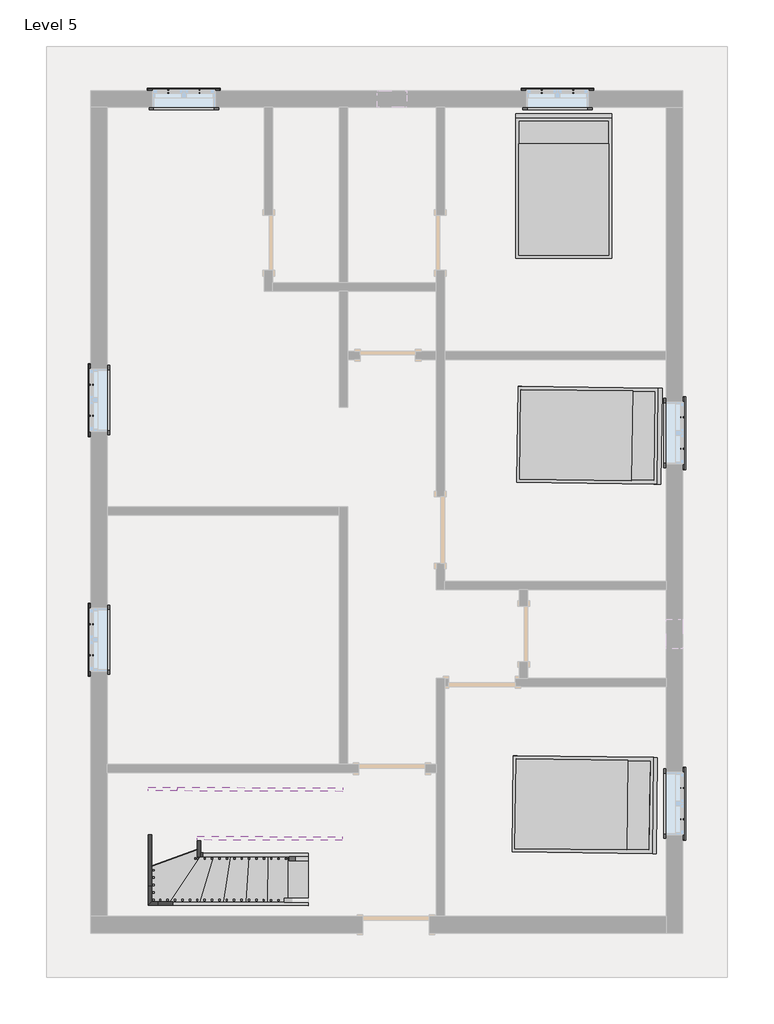
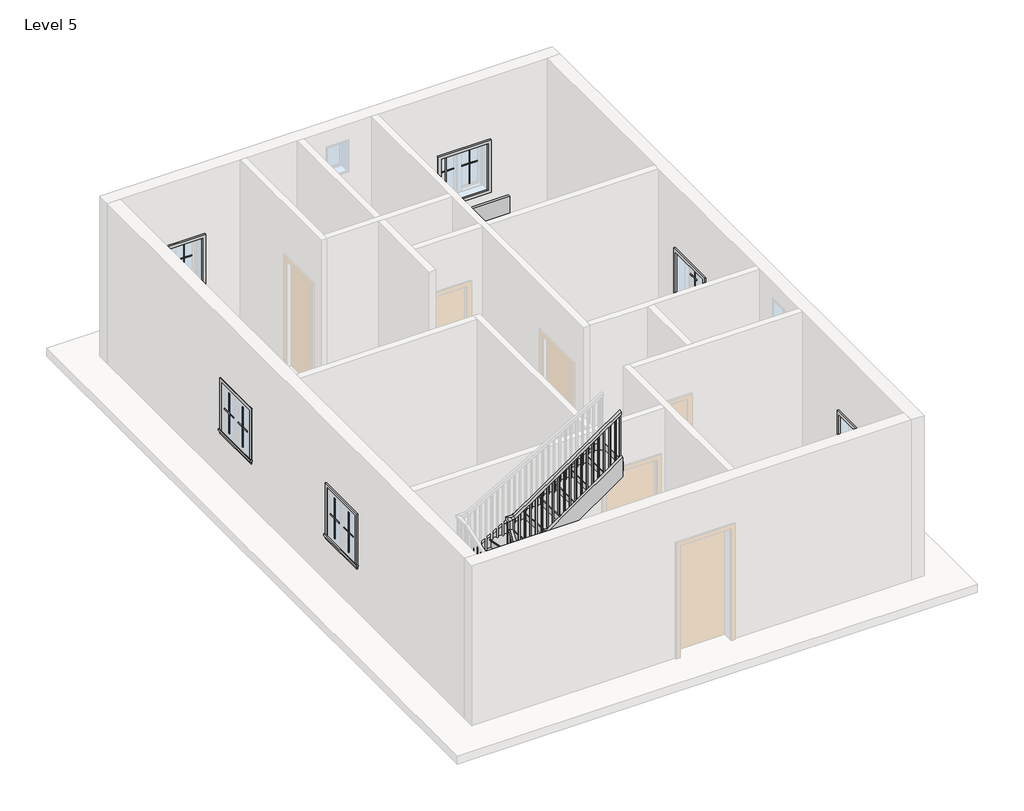
# One storey, part 3 of 3: 24 proxies, 9 members, 3 furniture elements, 1 railing, 1 stair flight.
"""IFC4 building model written with IfcOpenShell, lengths in millimetres."""

from ifc_helpers import new_model, si_unit, frame, origin, place, context, project, spatial, polyline, outline, extrude, faceted_brep, transform, mapped, element, save
from components import muntin_pattern_2x2_muntin_pattern_2x2_b3fe6957, muntin_pattern_2x2_muntin_pattern_2x2_3e0ecaf2, trim_window_exterior_flat_with_sill_41619996, trim_window_interior_flat_picture_frame_51c85655, bed_17739_bed_17739_15c61121, stair_flight_765c7f0f

model = new_model("IFC4")

# Units and contexts
model_context = context("Model", 3, world=origin())
ifc_project = project(units=[si_unit("LENGTHUNIT", "METRE", prefix="MILLI")], contexts=[model_context])

# Site, building, storey
site = spatial("IfcSite", under=ifc_project)
building = spatial("IfcBuilding", under=site)
storey = spatial("IfcBuildingStorey", under=building, Name="Level 5", Elevation=9601.2)

# Proxies
placement = place(None, origin())
muntin_pattern_2x2_muntin_pattern_2x2_shape = muntin_pattern_2x2_muntin_pattern_2x2_b3fe6957(model_context)
element("IfcBuildingElementProxy", 1, Name="Muntin Pattern_2x2 : Muntin Pattern_2x2", ObjectType="Muntin Pattern_2x2 : Muntin Pattern_2x2", at=placement, inside=storey, context=model_context, shape_type="MappedRepresentation", body=[
    mapped(muntin_pattern_2x2_muntin_pattern_2x2_shape, transform((873.7257686, 6321.6571212, 10585.45), x_axis=(1.0, 0.0, 0.0), y_axis=(0.0, 1.0, 0.0), z_axis=(0.0, 0.0, 1.0))),
])
element("IfcBuildingElementProxy", 2, Name="Muntin Pattern_2x2 : Muntin Pattern_2x2", ObjectType="Muntin Pattern_2x2 : Muntin Pattern_2x2", at=placement, inside=storey, context=model_context, shape_type="MappedRepresentation", body=[
    mapped(muntin_pattern_2x2_muntin_pattern_2x2_shape, transform((2802.5382686, 1840.1446212, 10585.45), x_axis=(0.0, -1.0, 0.0), y_axis=(1.0, 0.0, 0.0), z_axis=(0.0, 0.0, 1.0))),
])
element("IfcBuildingElementProxy", 3, Name="Muntin Pattern_2x2 : Muntin Pattern_2x2", ObjectType="Muntin Pattern_2x2 : Muntin Pattern_2x2", at=placement, inside=storey, context=model_context, shape_type="MappedRepresentation", body=[
    mapped(muntin_pattern_2x2_muntin_pattern_2x2_shape, transform((2802.5382686, -3255.7303788, 10585.45), x_axis=(0.0, -1.0, 0.0), y_axis=(1.0, 0.0, 0.0), z_axis=(0.0, 0.0, 1.0))),
])
element("IfcBuildingElementProxy", 4, Name="Muntin Pattern_2x2 : Muntin Pattern_2x2", ObjectType="Muntin Pattern_2x2 : Muntin Pattern_2x2", at=placement, inside=storey, context=model_context, shape_type="MappedRepresentation", body=[
    mapped(muntin_pattern_2x2_muntin_pattern_2x2_shape, transform((-4263.4242314, 6321.6571212, 10585.45), x_axis=(1.0, 0.0, 0.0), y_axis=(0.0, 1.0, 0.0), z_axis=(0.0, 0.0, 1.0))),
])
element("IfcBuildingElementProxy", 5, Name="Muntin Pattern_2x2 : Muntin Pattern_2x2", ObjectType="Muntin Pattern_2x2 : Muntin Pattern_2x2", at=placement, inside=storey, context=model_context, shape_type="MappedRepresentation", body=[
    mapped(muntin_pattern_2x2_muntin_pattern_2x2_shape, transform((-5319.1117314, 1863.8332318, 10585.45), x_axis=(0.0, 1.0, 0.0), y_axis=(-1.0, 0.0, 0.0), z_axis=(0.0, 0.0, 1.0))),
])
element("IfcBuildingElementProxy", 6, Name="Muntin Pattern_2x2 : Muntin Pattern_2x2", ObjectType="Muntin Pattern_2x2 : Muntin Pattern_2x2", at=placement, inside=storey, context=model_context, shape_type="MappedRepresentation", body=[
    mapped(muntin_pattern_2x2_muntin_pattern_2x2_shape, transform((-5319.1117314, -1431.8167682, 10585.45), x_axis=(0.0, 1.0, 0.0), y_axis=(-1.0, 0.0, 0.0), z_axis=(0.0, 0.0, 1.0))),
])
muntin_pattern_2x2_muntin_pattern_2x2_2_shape = muntin_pattern_2x2_muntin_pattern_2x2_3e0ecaf2(model_context)
element("IfcBuildingElementProxy", 7, Name="Muntin Pattern_2x2 : Muntin Pattern_2x2", ObjectType="Muntin Pattern_2x2 : Muntin Pattern_2x2", at=placement, inside=storey, context=model_context, shape_type="MappedRepresentation", body=[
    mapped(muntin_pattern_2x2_muntin_pattern_2x2_2_shape, transform((1302.3507686, 6321.6571212, 10585.45), x_axis=(-1.0, 0.0, 0.0), y_axis=(0.0, -1.0, 0.0), z_axis=(0.0, 0.0, 1.0))),
])
element("IfcBuildingElementProxy", 8, Name="Muntin Pattern_2x2 : Muntin Pattern_2x2", ObjectType="Muntin Pattern_2x2 : Muntin Pattern_2x2", at=placement, inside=storey, context=model_context, shape_type="MappedRepresentation", body=[
    mapped(muntin_pattern_2x2_muntin_pattern_2x2_2_shape, transform((2802.5382686, 1411.5196212, 10585.45), x_axis=(0.0, 1.0, 0.0), y_axis=(-1.0, 0.0, 0.0), z_axis=(0.0, 0.0, 1.0))),
])
element("IfcBuildingElementProxy", 9, Name="Muntin Pattern_2x2 : Muntin Pattern_2x2", ObjectType="Muntin Pattern_2x2 : Muntin Pattern_2x2", at=placement, inside=storey, context=model_context, shape_type="MappedRepresentation", body=[
    mapped(muntin_pattern_2x2_muntin_pattern_2x2_2_shape, transform((2802.5382686, -3684.3553788, 10585.45), x_axis=(0.0, 1.0, 0.0), y_axis=(-1.0, 0.0, 0.0), z_axis=(0.0, 0.0, 1.0))),
])
element("IfcBuildingElementProxy", 10, Name="Muntin Pattern_2x2 : Muntin Pattern_2x2", ObjectType="Muntin Pattern_2x2 : Muntin Pattern_2x2", at=placement, inside=storey, context=model_context, shape_type="MappedRepresentation", body=[
    mapped(muntin_pattern_2x2_muntin_pattern_2x2_2_shape, transform((-3834.7992314, 6321.6571212, 10585.45), x_axis=(-1.0, 0.0, 0.0), y_axis=(0.0, -1.0, 0.0), z_axis=(0.0, 0.0, 1.0))),
])
element("IfcBuildingElementProxy", 11, Name="Muntin Pattern_2x2 : Muntin Pattern_2x2", ObjectType="Muntin Pattern_2x2 : Muntin Pattern_2x2", at=placement, inside=storey, context=model_context, shape_type="MappedRepresentation", body=[
    mapped(muntin_pattern_2x2_muntin_pattern_2x2_2_shape, transform((-5319.1117314, 2292.4582318, 10585.45), x_axis=(0.0, -1.0, 0.0), y_axis=(1.0, 0.0, 0.0), z_axis=(0.0, 0.0, 1.0))),
])
element("IfcBuildingElementProxy", 12, Name="Muntin Pattern_2x2 : Muntin Pattern_2x2", ObjectType="Muntin Pattern_2x2 : Muntin Pattern_2x2", at=placement, inside=storey, context=model_context, shape_type="MappedRepresentation", body=[
    mapped(muntin_pattern_2x2_muntin_pattern_2x2_2_shape, transform((-5319.1117314, -1003.1917682, 10585.45), x_axis=(0.0, -1.0, 0.0), y_axis=(1.0, 0.0, 0.0), z_axis=(0.0, 0.0, 1.0))),
])
trim_window_exterior_flat_with_sill_shape = trim_window_exterior_flat_with_sill_41619996(model_context)
element("IfcBuildingElementProxy", 13, Name="Trim-Window-Exterior-Flat : with Sill", ObjectType="Trim-Window-Exterior-Flat : with Sill", at=placement, inside=storey, context=model_context, shape_type="MappedRepresentation", body=[
    mapped(trim_window_exterior_flat_with_sill_shape, transform((1088.0382686, 6331.1821212, 11430.0), x_axis=(-1.0, 0.0, 0.0), y_axis=(0.0, 0.0, 1.0), z_axis=(0.0, 1.0, 0.0))),
])
element("IfcBuildingElementProxy", 14, Name="Trim-Window-Exterior-Flat : with Sill", ObjectType="Trim-Window-Exterior-Flat : with Sill", at=placement, inside=storey, context=model_context, shape_type="MappedRepresentation", body=[
    mapped(trim_window_exterior_flat_with_sill_shape, transform((2812.0632686, 1625.8321212, 11430.0), x_axis=(0.0, 1.0, 0.0), y_axis=(0.0, 0.0, 1.0), z_axis=(1.0, 0.0, 0.0))),
])
element("IfcBuildingElementProxy", 15, Name="Trim-Window-Exterior-Flat : with Sill", ObjectType="Trim-Window-Exterior-Flat : with Sill", at=placement, inside=storey, context=model_context, shape_type="MappedRepresentation", body=[
    mapped(trim_window_exterior_flat_with_sill_shape, transform((2812.0632686, -3470.0428788, 11430.0), x_axis=(0.0, 1.0, 0.0), y_axis=(0.0, 0.0, 1.0), z_axis=(1.0, 0.0, 0.0))),
])
element("IfcBuildingElementProxy", 16, Name="Trim-Window-Exterior-Flat : with Sill", ObjectType="Trim-Window-Exterior-Flat : with Sill", at=placement, inside=storey, context=model_context, shape_type="MappedRepresentation", body=[
    mapped(trim_window_exterior_flat_with_sill_shape, transform((-4049.1117314, 6331.1821212, 11430.0), x_axis=(-1.0, 0.0, 0.0), y_axis=(0.0, 0.0, 1.0), z_axis=(0.0, 1.0, 0.0))),
])
element("IfcBuildingElementProxy", 17, Name="Trim-Window-Exterior-Flat : with Sill", ObjectType="Trim-Window-Exterior-Flat : with Sill", at=placement, inside=storey, context=model_context, shape_type="MappedRepresentation", body=[
    mapped(trim_window_exterior_flat_with_sill_shape, transform((-5328.6367314, 2078.1457318, 11430.0), x_axis=(0.0, -1.0, 0.0), y_axis=(0.0, 0.0, 1.0), z_axis=(-1.0, 0.0, 0.0))),
])
element("IfcBuildingElementProxy", 18, Name="Trim-Window-Exterior-Flat : with Sill", ObjectType="Trim-Window-Exterior-Flat : with Sill", at=placement, inside=storey, context=model_context, shape_type="MappedRepresentation", body=[
    mapped(trim_window_exterior_flat_with_sill_shape, transform((-5328.6367314, -1217.5042682, 11430.0), x_axis=(0.0, -1.0, 0.0), y_axis=(0.0, 0.0, 1.0), z_axis=(-1.0, 0.0, 0.0))),
])
trim_window_interior_flat_picture_frame_shape = trim_window_interior_flat_picture_frame_51c85655(model_context)
element("IfcBuildingElementProxy", 19, Name="Trim-Window-Interior-Flat : Picture Frame", ObjectType="Trim-Window-Interior-Flat : Picture Frame", at=placement, inside=storey, context=model_context, shape_type="MappedRepresentation", body=[
    mapped(trim_window_interior_flat_picture_frame_shape, transform((1088.0382686, 6102.5821212, 11430.0), x_axis=(1.0, 0.0, 0.0), y_axis=(0.0, 0.0, 1.0), z_axis=(0.0, -1.0, 0.0))),
])
element("IfcBuildingElementProxy", 20, Name="Trim-Window-Interior-Flat : Picture Frame", ObjectType="Trim-Window-Interior-Flat : Picture Frame", at=placement, inside=storey, context=model_context, shape_type="MappedRepresentation", body=[
    mapped(trim_window_interior_flat_picture_frame_shape, transform((2583.4632686, 1625.8321212, 11430.0), x_axis=(0.0, -1.0, 0.0), y_axis=(0.0, 0.0, 1.0), z_axis=(-1.0, 0.0, 0.0))),
])
element("IfcBuildingElementProxy", 21, Name="Trim-Window-Interior-Flat : Picture Frame", ObjectType="Trim-Window-Interior-Flat : Picture Frame", at=placement, inside=storey, context=model_context, shape_type="MappedRepresentation", body=[
    mapped(trim_window_interior_flat_picture_frame_shape, transform((2583.4632686, -3470.0428788, 11430.0), x_axis=(0.0, -1.0, 0.0), y_axis=(0.0, 0.0, 1.0), z_axis=(-1.0, 0.0, 0.0))),
])
element("IfcBuildingElementProxy", 22, Name="Trim-Window-Interior-Flat : Picture Frame", ObjectType="Trim-Window-Interior-Flat : Picture Frame", at=placement, inside=storey, context=model_context, shape_type="MappedRepresentation", body=[
    mapped(trim_window_interior_flat_picture_frame_shape, transform((-4049.1117314, 6102.5821212, 11430.0), x_axis=(1.0, 0.0, 0.0), y_axis=(0.0, 0.0, 1.0), z_axis=(0.0, -1.0, 0.0))),
])
element("IfcBuildingElementProxy", 23, Name="Trim-Window-Interior-Flat : Picture Frame", ObjectType="Trim-Window-Interior-Flat : Picture Frame", at=placement, inside=storey, context=model_context, shape_type="MappedRepresentation", body=[
    mapped(trim_window_interior_flat_picture_frame_shape, transform((-5100.0367314, 2078.1457318, 11430.0), x_axis=(0.0, 1.0, 0.0), y_axis=(0.0, 0.0, 1.0), z_axis=(1.0, 0.0, 0.0))),
])
element("IfcBuildingElementProxy", 24, Name="Trim-Window-Interior-Flat : Picture Frame", ObjectType="Trim-Window-Interior-Flat : Picture Frame", at=placement, inside=storey, context=model_context, shape_type="MappedRepresentation", body=[
    mapped(trim_window_interior_flat_picture_frame_shape, transform((-5100.0367314, -1217.5042682, 11430.0), x_axis=(0.0, 1.0, 0.0), y_axis=(0.0, 0.0, 1.0), z_axis=(1.0, 0.0, 0.0))),
])

# Furniture
bed_17739_bed_17739_shape = bed_17739_bed_17739_15c61121(model_context)
element("IfcFurniture", 25, ObjectType="Bed_17739 : Bed_17739", at=placement, inside=storey, context=model_context, shape_type="MappedRepresentation", body=[
    mapped(bed_17739_bed_17739_shape, transform((1173.7632686, 4997.6821212, 9601.2), x_axis=(1.0, 0.0, 0.0), y_axis=(0.0, 1.0, 0.0), z_axis=(0.0, 0.0, 1.0))),
])
element("IfcFurniture", 26, ObjectType="Bed_17739 : Bed_17739", at=placement, inside=storey, context=model_context, shape_type="MappedRepresentation", body=[
    mapped(bed_17739_bed_17739_shape, transform((1503.3372561, 1596.4447738, 9601.2), x_axis=(-0.012740965827000846, -0.9999188306006619, 0.0), y_axis=(0.9999188306006619, -0.012740965827000846, 0.0), z_axis=(0.0, 0.0, 1.0))),
])
element("IfcFurniture", 27, ObjectType="Bed_17739 : Bed_17739", at=placement, inside=storey, context=model_context, shape_type="MappedRepresentation", body=[
    mapped(bed_17739_bed_17739_shape, transform((1438.6034215, -3483.9063624, 9601.2), x_axis=(-0.012740965827007402, -0.9999188306006618, 0.0), y_axis=(0.9999188306006618, -0.012740965827007402, 0.0), z_axis=(0.0, 0.0, 1.0))),
])

# Members
element("IfcMember", 28, ObjectType="Stringer - 2\" Width", at=placement, inside=storey, context=model_context, shape_type="SweptSolid", body=[
    extrude(outline(polyline([(-105.6436802, -202.41926), (0.0, 0.0), (2328.0658822, 0.0), (2168.9891534, -304.7999999), (90.5236019, -304.7999999), (-105.6436802, -202.41926)])), frame((-2342.1993001, -4876.8012848, 9829.5290257), z_axis=(0.0033835818014385675, 0.9999942756707125, 0.0), x_axis=(-0.8865193579369285, 0.002999627936996439, 0.46268178074713046)), (0.0, 0.0, 1.0), 50.8),
])
element("IfcMember", 29, ObjectType="Stringer - 2\" Width", at=placement, inside=storey, context=model_context, shape_type="SweptSolid", body=[
    extrude(outline(polyline([(-4405.9028852, -4819.0182441), (-4406.0747712, -4869.8179533), (-4542.6986856, -4869.3556725), (-4491.7270905, -4818.7278493), (-4405.9028852, -4819.0182441)])), frame((0.0, 0.0, 10562.8681426), z_axis=(0.0, 0.0, 1.0), x_axis=(1.0, 0.0, 0.0)), (0.0, 0.0, 1.0), 343.8145513),
])
element("IfcMember", 30, ObjectType="Stringer - 2\" Width", at=placement, inside=storey, context=model_context, shape_type="SweptSolid", body=[
    extrude(outline(polyline([(-4491.7270905, -4818.7278493), (-4542.6986856, -4869.3556725), (-4541.8102896, -4606.7963526), (-4491.0105804, -4606.9682386), (-4491.7270905, -4818.7278493)])), frame((0.0, 0.0, 10562.8681426), z_axis=(0.0, 0.0, 1.0), x_axis=(1.0, 0.0, 0.0)), (0.0, 0.0, 1.0), 343.8145513),
])
element("IfcMember", 31, ObjectType="Stringer - 2\" Width", at=placement, inside=storey, context=model_context, shape_type="SweptSolid", body=[
    extrude(outline(polyline([(109.7110974, -325.8403301), (0.0, 0.0), (1383.9510961, 0.0), (1489.930143, -314.7561954), (1457.0104275, -325.8403301), (109.7110974, -325.8403301)])), frame((-4491.0105804, -4606.9682386, 10562.8681426), z_axis=(-0.9999942756707125, 0.003383581801438881, 0.0), x_axis=(0.0032066921171017425, 0.9477157489074123, 0.3190996339680272)), (0.0, 0.0, 1.0), 50.8),
])
element("IfcMember", 32, ObjectType="Stringer - 2\" Width", at=placement, inside=storey, context=model_context, shape_type="SweptSolid", body=[
    extrude(outline(polyline([(-4537.3723845, -3295.2041032), (-4537.2004986, -3244.404394), (-4139.0142012, -3245.7516976), (-4139.1860871, -3296.5514068), (-4537.3723845, -3295.2041032)])), frame((0.0, 0.0, 11014.9918365), z_axis=(0.0, 0.0, 1.0), x_axis=(1.0, 0.0, 0.0)), (0.0, 0.0, 1.0), 321.6135804),
])
element("IfcMember", 33, ObjectType="Stringer - 2\" Width", at=placement, inside=storey, context=model_context, shape_type="SweptSolid", body=[
    extrude(outline(polyline([(-111.9549294, -160.635527), (0.0, 0.0), (1800.2454177, 0.0), (1587.8150598, -304.8000001), (94.8955973, -304.8), (-111.9549294, -160.635527)])), frame((-2339.9228929, -4204.0248458, 9797.0000989), z_axis=(0.0033835818014388334, 0.9999942756707125, 0.0), x_axis=(-0.82040105359797, 0.0027759099650580487, 0.5717817814334475)), (0.0, 0.0, 1.0), 50.8),
])
element("IfcMember", 34, ObjectType="Stringer - 2\" Width", at=placement, inside=storey, context=model_context, shape_type="SweptSolid", body=[
    extrude(outline(polyline([(438.5777673, -304.8), (2.5808594, -1.7936294), (3.8273846, 0.0), (400.5684618, 0.0), (819.8223258, -291.370396), (810.4891046, -304.8000001), (438.5777673, -304.8)])), frame((-3816.8461303, -4199.0275266, 10487.0862902), z_axis=(-0.9999942756707126, 0.00338358180143736, 0.0), x_axis=(0.0019309727886813012, 0.5706856959500531, 0.8211663094538725)), (0.0, 0.0, 1.0), 50.8),
])
element("IfcMember", 35, ObjectType="Stringer - 2\" Width", at=placement, inside=storey, context=model_context, shape_type="SweptSolid", body=[
    extrude(outline(polyline([(213.8292849, -304.8), (0.0, 0.0), (2440.5867528, 0.0), (2654.4160377, -304.8), (213.8292849, -304.8)])), frame((-3866.8723527, -3970.2569493, 10954.2535021), z_axis=(0.003383581801438697, 0.9999942756707126, 0.0), x_axis=(0.8186346554264393, -0.0027699331781375542, 0.5743079560697587)), (0.0, 0.0, 1.0), 50.8),
])
element("IfcMember", 36, ObjectType="Stringer - 2\" Width", at=placement, inside=storey, context=model_context, shape_type="SweptSolid", body=[
    extrude(outline(polyline([(162.5062199, -277.5374274), (0.0, 0.0), (2633.4595913, 1e-07), (2795.9658112, -277.5374274), (162.5062199, -277.5374274)])), frame((-4139.1860871, -3296.5514068, 11014.9918365), z_axis=(0.003383581801438589, 0.9999942756707125, 0.0), x_axis=(0.8629481327443966, -0.002919872311849943, 0.5052840731100098)), (0.0, 0.0, 1.0), 50.8),
])

# Railing
element("IfcRailing", 37, ObjectType="Handrail - Rectangular", at=placement, inside=storey, context=model_context, shape_type="SolidModel", body=[
    faceted_brep([(-2340.0947789, -4254.824555, 10684.9333333), (-2340.0947789, -4254.824555, 10623.5023206), (-2339.9228929, -4204.0248458, 10623.5023206), (-2339.9228929, -4204.0248458, 10684.9333333), (-3791.6181617, -4249.9131788, 11671.9092848), (-3842.4178709, -4249.7412929, 11645.0199762), (-3842.2459849, -4198.9415837, 11645.0199762), (-3791.4462757, -4199.1134696, 11671.9092848), (-1868.5796854, -3875.4177931, 13563.6), (-1868.7515713, -3926.2175023, 13563.6), (-1868.7515713, -3926.2175023, 13501.938507), (-1868.5796854, -3875.4177931, 13501.938507), (-3774.5418549, -3868.9687773, 12190.645528), (-3790.329017, -3868.9153598, 12241.445528), (-3774.7137409, -3919.7684865, 12190.645528), (-3790.500903, -3919.715069, 12241.445528), (-3791.6181617, -4249.9131788, 11888.2182666), (-3842.4178709, -4249.7412929, 11837.4182666), (-3842.2459849, -4198.9415837, 11837.4182666), (-3791.4462757, -4199.1134696, 11888.2182666), (-3918.6174347, -4249.4834639, 11888.2182666), (-3918.6174347, -4249.4834639, 11837.4182666), (-3867.6458395, -4198.8556407, 11837.4182666), (-3867.6458395, -4198.8556407, 11888.2182666), (-3918.1877198, -4122.4841909, 11888.2182666), (-3918.0978567, -4095.9257757, 11837.4182666), (-3867.2981475, -4096.0976616, 11837.4182666), (-3867.3880106, -4122.6560769, 11888.2182666), (-3917.7580049, -3995.4849179, 12070.959003), (-3917.586119, -3944.6852087, 12055.0400838), (-3866.7864097, -3944.8570947, 12055.0400838), (-3866.9582957, -3995.6568039, 12070.959003), (-3917.7580049, -3995.4849179, 12241.445528), (-3917.586119, -3944.6852087, 12190.645528), (-3866.7864097, -3944.8570947, 12190.645528), (-3866.9582957, -3995.6568039, 12241.445528), (-3917.32829, -3868.4856449, 12241.445528), (-3917.32829, -3868.4856449, 12190.645528), (-3866.7004668, -3919.4572401, 12190.645528), (-3866.7004668, -3919.4572401, 12241.445528)], [[[0, 1, 2, 3]], [[1, 0, 4, 5]], [[2, 1, 5, 6]], [[3, 2, 6, 7]], [[0, 3, 7, 4]], [[8, 9, 10, 11]], [[12, 13, 8, 11]], [[14, 12, 11, 10]], [[15, 14, 10, 9]], [[13, 15, 9, 8]], [[5, 4, 16, 17]], [[6, 5, 17, 18]], [[7, 6, 18, 19]], [[4, 7, 19, 16]], [[17, 16, 20, 21]], [[18, 17, 21, 22]], [[19, 18, 22, 23]], [[16, 19, 23, 20]], [[21, 20, 24, 25]], [[22, 21, 25, 26]], [[23, 22, 26, 27]], [[20, 23, 27, 24]], [[25, 24, 28, 29]], [[26, 25, 29, 30]], [[27, 26, 30, 31]], [[24, 27, 31, 28]], [[29, 28, 32, 33]], [[30, 29, 33, 34]], [[31, 30, 34, 35]], [[28, 31, 35, 32]], [[33, 32, 36, 37]], [[34, 33, 37, 38]], [[35, 34, 38, 39]], [[32, 35, 39, 36]], [[37, 36, 13, 12]], [[38, 37, 12, 14]], [[39, 38, 14, 15]], [[36, 39, 15, 13]]]),
    extrude(outline(polyline([(222.0468824, -19.0499999), (235.1531175, 0.0), (1186.7159363, 0.0), (1186.7159363, -19.0499999), (222.0468824, -19.0499999)])), frame((-1971.1826027, -3909.9958257, 13666.582603), z_axis=(0.0033835818014386967, 0.9999942756707125, 0.0), x_axis=(0.0, 0.0, -1.0)), (0.0, 0.0, 1.0), 19.05),
    extrude(outline(polyline([(222.0468825, -19.0499999), (235.1531175, 0.0), (1116.8160159, 0.0), (1116.8160159, -19.0499999), (222.0468825, -19.0499999)])), frame((-2072.7820211, -3909.6520537, 13596.6826826), z_axis=(0.0033835818014386967, 0.9999942756707125, 0.0), x_axis=(0.0, 0.0, -1.0)), (0.0, 0.0, 1.0), 19.05),
    extrude(outline(polyline([(222.0468825, -19.0499999), (235.1531176, 0.0), (1216.2494289, 0.0), (1216.2494289, -19.0499999), (222.0468825, -19.0499999)])), frame((-2174.3814395, -3909.3082818, 13526.7827622), z_axis=(0.0033835818014386967, 0.9999942756707125, 0.0), x_axis=(0.0, 0.0, -1.0)), (0.0, 0.0, 1.0), 19.05),
    extrude(outline(polyline([(222.0468825, -19.05), (235.1531175, 0.0), (1146.3495084, 0.0), (1146.3495084, -19.05), (222.0468825, -19.05)])), frame((-2275.980858, -3908.9645099, 13456.8828417), z_axis=(0.0033835818014386967, 0.9999942756707125, 0.0), x_axis=(0.0, 0.0, -1.0)), (0.0, 0.0, 1.0), 19.05),
    extrude(outline(polyline([(222.0468825, -19.05), (235.1531176, 0.0), (1076.449588, 0.0), (1076.449588, -19.05), (222.0468825, -19.05)])), frame((-2377.5802764, -3908.620738, 13386.9829213), z_axis=(0.0033835818014386967, 0.9999942756707125, 0.0), x_axis=(0.0, 0.0, -1.0)), (0.0, 0.0, 1.0), 19.05),
    extrude(outline(polyline([(222.0468824, -19.05), (235.1531175, 0.0), (1175.8830008, 0.0), (1175.8830008, -19.05), (222.0468824, -19.05)])), frame((-2479.1796948, -3908.2769661, 13317.0830008), z_axis=(0.0033835818014386967, 0.9999942756707125, 0.0), x_axis=(0.0, 0.0, -1.0)), (0.0, 0.0, 1.0), 19.05),
    extrude(outline(polyline([(222.0468825, -19.05), (235.1531176, 0.0), (1105.9830804, 0.0), (1105.9830804, -19.05), (222.0468825, -19.05)])), frame((-2580.7791132, -3907.9331942, 13247.1830804), z_axis=(0.0033835818014386967, 0.9999942756707125, 0.0), x_axis=(0.0, 0.0, -1.0)), (0.0, 0.0, 1.0), 19.05),
    extrude(outline(polyline([(222.0468824, -19.05), (235.1531175, 0.0), (1036.0831599, 0.0), (1036.0831599, -19.05), (222.0468824, -19.05)])), frame((-2682.3785316, -3907.5894223, 13177.2831599), z_axis=(0.0033835818014386967, 0.9999942756707125, 0.0), x_axis=(0.0, 0.0, -1.0)), (0.0, 0.0, 1.0), 19.05),
    extrude(outline(polyline([(222.0468825, -19.05), (235.1531176, 0.0), (1135.5165728, 0.0), (1135.5165728, -19.05), (222.0468825, -19.05)])), frame((-2783.97795, -3907.2456504, 13107.3832395), z_axis=(0.0033835818014386967, 0.9999942756707125, 0.0), x_axis=(0.0, 0.0, -1.0)), (0.0, 0.0, 1.0), 19.05),
    extrude(outline(polyline([(222.0468824, -19.0499999), (235.1531175, 0.0), (1065.6166523, 0.0), (1065.6166523, -19.0499999), (222.0468824, -19.0499999)])), frame((-2885.5773684, -3906.9018785, 13037.483319), z_axis=(0.0033835818014386967, 0.9999942756707125, 0.0), x_axis=(0.0, 0.0, -1.0)), (0.0, 0.0, 1.0), 19.05),
    extrude(outline(polyline([(222.0468825, -19.0499999), (235.1531176, 0.0), (995.7167319, 0.0), (995.7167319, -19.0499999), (222.0468825, -19.0499999)])), frame((-2987.1767868, -3906.5581065, 12967.5833986), z_axis=(0.0033835818014386967, 0.9999942756707125, 0.0), x_axis=(0.0, 0.0, -1.0)), (0.0, 0.0, 1.0), 19.05),
    extrude(outline(polyline([(222.0468824, -19.0499999), (235.1531175, 0.0), (1095.1501448, 0.0), (1095.1501448, -19.0499999), (222.0468824, -19.0499999)])), frame((-3088.7762052, -3906.2143346, 12897.6834781), z_axis=(0.0033835818014386967, 0.9999942756707125, 0.0), x_axis=(0.0, 0.0, -1.0)), (0.0, 0.0, 1.0), 19.05),
    extrude(outline(polyline([(222.0468825, -19.0499999), (235.1531176, 0.0), (1025.2502244, 0.0), (1025.2502244, -19.0499999), (222.0468825, -19.0499999)])), frame((-3190.3756236, -3905.8705627, 12827.7835577), z_axis=(0.0033835818014386967, 0.9999942756707125, 0.0), x_axis=(0.0, 0.0, -1.0)), (0.0, 0.0, 1.0), 19.05),
    extrude(outline(polyline([(222.0468824, -19.0499999), (235.1531175, 0.0), (1124.6836372, 0.0), (1124.6836372, -19.0499999), (222.0468824, -19.0499999)])), frame((-3291.975042, -3905.5267908, 12757.8836372), z_axis=(0.0033835818014386967, 0.9999942756707125, 0.0), x_axis=(0.0, 0.0, -1.0)), (0.0, 0.0, 1.0), 19.05),
    extrude(outline(polyline([(222.0468825, -19.0499999), (235.1531176, 0.0), (1054.7837168, 0.0), (1054.7837168, -19.0499999), (222.0468825, -19.0499999)])), frame((-3393.5744604, -3905.1830189, 12687.9837168), z_axis=(0.0033835818014386967, 0.9999942756707125, 0.0), x_axis=(0.0, 0.0, -1.0)), (0.0, 0.0, 1.0), 19.05),
    extrude(outline(polyline([(222.0468824, -19.05), (235.1531175, 0.0), (984.8837963, 0.0), (984.8837963, -19.05), (222.0468824, -19.05)])), frame((-3495.1738789, -3904.839247, 12618.0837963), z_axis=(0.0033835818014386967, 0.9999942756707125, 0.0), x_axis=(0.0, 0.0, -1.0)), (0.0, 0.0, 1.0), 19.05),
    extrude(outline(polyline([(222.0468825, -19.05), (235.1531176, 0.0), (1084.3172092, 0.0), (1084.3172092, -19.05), (222.0468825, -19.05)])), frame((-3596.7732973, -3904.4954751, 12548.1838759), z_axis=(0.0033835818014386967, 0.9999942756707125, 0.0), x_axis=(0.0, 0.0, -1.0)), (0.0, 0.0, 1.0), 19.05),
    extrude(outline(polyline([(222.0468824, -19.05), (235.1531175, 0.0), (1014.4172887, 0.0), (1014.4172887, -19.05), (222.0468824, -19.05)])), frame((-3698.3727157, -3904.1517032, 12478.2839554), z_axis=(0.0033835818014386967, 0.9999942756707125, 0.0), x_axis=(0.0, 0.0, -1.0)), (0.0, 0.0, 1.0), 19.05),
    extrude(outline(polyline([(222.0468825, -19.05), (235.1531175, 0.0), (1113.8507017, 0.0), (1113.8507017, -19.05), (222.0468825, -19.05)])), frame((-3799.9721341, -3903.8079313, 12408.384035), z_axis=(0.0033835818014386967, 0.9999942756707125, 0.0), x_axis=(0.0, 0.0, -1.0)), (0.0, 0.0, 1.0), 19.05),
    extrude(outline(polyline([(-3882.6076045, -3928.9284712), (-3901.6574955, -3928.8640139), (-3901.5930382, -3909.814123), (-3882.5431473, -3909.8785802), (-3882.6076045, -3928.9284712)])), frame((0.0, 0.0, 11125.2), z_axis=(0.0, 0.0, 1.0), x_axis=(1.0, 0.0, 0.0)), (0.0, 0.0, 1.0), 1065.445528),
    extrude(outline(polyline([(214.8944448, -19.05), (242.3055552, 0.0), (1218.1289753, 0.0), (1218.1289753, -19.05), (214.8944448, -19.05)])), frame((-3882.9513764, -4030.5278896, 12173.995642), z_axis=(-0.9999942756707125, 0.0033835818014373593, 0.0), x_axis=(0.0, 0.0, -1.0)), (0.0, 0.0, 1.0), 19.05),
    extrude(outline(polyline([(214.8944448, -19.05), (242.3055552, 0.0), (1071.9363862, 0.0), (1071.9363862, -19.05), (214.8944448, -19.05)])), frame((-3883.2951483, -4132.127308, 12027.8030529), z_axis=(-0.9999942756707125, 0.0033835818014373593, 0.0), x_axis=(0.0, 0.0, -1.0)), (0.0, 0.0, 1.0), 19.05),
    extrude(outline(polyline([(-3854.4429379, -4214.7754049), (-3854.5073951, -4233.8252959), (-3873.5572861, -4233.7608386), (-3873.4928289, -4214.7109477), (-3854.4429379, -4214.7754049)])), frame((0.0, 0.0, 10786.5333333), z_axis=(0.0, 0.0, 1.0), x_axis=(1.0, 0.0, 0.0)), (0.0, 0.0, 1.0), 1050.8849333),
    extrude(outline(polyline([(235.0765695, -19.05), (222.1234305, 0.0), (1202.0700381, 0.0), (1202.0700381, -19.05), (235.0765695, -19.05)])), frame((-3771.9578677, -4234.1046105, 11819.2700381), z_axis=(0.003383581801438833, 0.9999942756707125, 0.0), x_axis=(0.0, 0.0, -1.0)), (0.0, 0.0, 1.0), 19.05),
    extrude(outline(polyline([(235.0765695, -19.05), (222.1234305, 0.0), (1132.9866297, 0.0), (1132.9866297, -19.05), (235.0765695, -19.05)])), frame((-3670.3584493, -4234.4483825, 11750.1866297), z_axis=(0.003383581801438833, 0.9999942756707125, 0.0), x_axis=(0.0, 0.0, -1.0)), (0.0, 0.0, 1.0), 19.05),
    extrude(outline(polyline([(235.0765695, -19.05), (222.1234305, 0.0), (1233.2365546, 0.0), (1233.2365546, -19.05), (235.0765695, -19.05)])), frame((-3568.7590309, -4234.7921544, 11681.1032213), z_axis=(0.003383581801438833, 0.9999942756707125, 0.0), x_axis=(0.0, 0.0, -1.0)), (0.0, 0.0, 1.0), 19.05),
    extrude(outline(polyline([(235.0765695, -19.05), (222.1234305, 0.0), (1164.1531462, 0.0), (1164.1531462, -19.05), (235.0765695, -19.05)])), frame((-3467.1596125, -4235.1359263, 11612.0198129), z_axis=(0.003383581801438833, 0.9999942756707125, 0.0), x_axis=(0.0, 0.0, -1.0)), (0.0, 0.0, 1.0), 19.05),
    extrude(outline(polyline([(235.0765695, -19.05), (222.1234305, 0.0), (1264.4030712, 0.0), (1264.4030712, -19.05), (235.0765695, -19.05)])), frame((-3365.5601941, -4235.4796982, 11542.9364045), z_axis=(0.003383581801438833, 0.9999942756707125, 0.0), x_axis=(0.0, 0.0, -1.0)), (0.0, 0.0, 1.0), 19.05),
    extrude(outline(polyline([(235.0765695, -19.0499999), (222.1234304, 0.0), (1195.3196628, 0.0), (1195.3196628, -19.0499999), (235.0765695, -19.0499999)])), frame((-3263.9607756, -4235.8234701, 11473.8529961), z_axis=(0.003383581801438833, 0.9999942756707125, 0.0), x_axis=(0.0, 0.0, -1.0)), (0.0, 0.0, 1.0), 19.05),
    extrude(outline(polyline([(235.0765695, -19.0499999), (222.1234304, 0.0), (1295.5695877, 0.0), (1295.5695877, -19.0499999), (235.0765695, -19.0499999)])), frame((-3162.3613572, -4236.167242, 11404.7695877), z_axis=(0.003383581801438833, 0.9999942756707125, 0.0), x_axis=(0.0, 0.0, -1.0)), (0.0, 0.0, 1.0), 19.05),
    extrude(outline(polyline([(235.0765695, -19.0499999), (222.1234304, 0.0), (1226.4861793, 0.0), (1226.4861793, -19.0499999), (235.0765695, -19.0499999)])), frame((-3060.7619388, -4236.5110139, 11335.6861793), z_axis=(0.003383581801438833, 0.9999942756707125, 0.0), x_axis=(0.0, 0.0, -1.0)), (0.0, 0.0, 1.0), 19.05),
    extrude(outline(polyline([(235.0765695, -19.0499999), (222.1234304, 0.0), (1157.4027709, 0.0), (1157.4027709, -19.0499999), (235.0765695, -19.0499999)])), frame((-2959.1625204, -4236.8547858, 11266.6027709), z_axis=(0.003383581801438833, 0.9999942756707125, 0.0), x_axis=(0.0, 0.0, -1.0)), (0.0, 0.0, 1.0), 19.05),
    extrude(outline(polyline([(235.0765695, -19.0499999), (222.1234304, 0.0), (1257.6526958, 0.0), (1257.6526958, -19.0499999), (235.0765695, -19.0499999)])), frame((-2857.563102, -4237.1985577, 11197.5193625), z_axis=(0.003383581801438833, 0.9999942756707125, 0.0), x_axis=(0.0, 0.0, -1.0)), (0.0, 0.0, 1.0), 19.05),
    extrude(outline(polyline([(235.0765695, -19.0499999), (222.1234304, 0.0), (1188.5692874, 0.0), (1188.5692874, -19.0499999), (235.0765695, -19.0499999)])), frame((-2755.9636836, -4237.5423297, 11128.4359541), z_axis=(0.003383581801438833, 0.9999942756707125, 0.0), x_axis=(0.0, 0.0, -1.0)), (0.0, 0.0, 1.0), 19.05),
    extrude(outline(polyline([(235.0765696, -19.05), (222.1234305, 0.0), (1119.4858791, 0.0), (1119.4858791, -19.05), (235.0765696, -19.05)])), frame((-2654.3642652, -4237.8861016, 11059.3525458), z_axis=(0.003383581801438833, 0.9999942756707125, 0.0), x_axis=(0.0, 0.0, -1.0)), (0.0, 0.0, 1.0), 19.05),
    extrude(outline(polyline([(235.0765696, -19.05), (222.1234305, 0.0), (1219.7358041, 0.0), (1219.7358041, -19.05), (235.0765696, -19.05)])), frame((-2552.7648468, -4238.2298735, 10990.2691374), z_axis=(0.003383581801438833, 0.9999942756707125, 0.0), x_axis=(0.0, 0.0, -1.0)), (0.0, 0.0, 1.0), 19.05),
    extrude(outline(polyline([(235.0765696, -19.05), (222.1234305, 0.0), (1150.6523957, 0.0), (1150.6523957, -19.05), (235.0765696, -19.05)])), frame((-2451.1654284, -4238.5736454, 10921.185729), z_axis=(0.003383581801438833, 0.9999942756707125, 0.0), x_axis=(0.0, 0.0, -1.0)), (0.0, 0.0, 1.0), 19.05),
    extrude(outline(polyline([(-3882.5216615, -3903.5286166), (-3901.5715525, -3903.4641593), (-3901.5070953, -3884.4142684), (-3882.4572043, -3884.4787256), (-3882.5216615, -3903.5286166)])), frame((0.0, 0.0, 11125.2), z_axis=(0.0, 0.0, 1.0), x_axis=(1.0, 0.0, 0.0)), (0.0, 0.0, 1.0), 1065.445528),
    extrude(outline(polyline([(-3883.574463, -4214.6768355), (-3883.6389202, -4233.7267264), (-3902.6888112, -4233.6622692), (-3902.624354, -4214.6123782), (-3883.574463, -4214.6768355)])), frame((0.0, 0.0, 10786.5333333), z_axis=(0.0, 0.0, 1.0), x_axis=(1.0, 0.0, 0.0)), (0.0, 0.0, 1.0), 1050.8849333),
    extrude(outline(polyline([(222.0468825, -19.0499999), (235.1531176, 0.0), (1244.1187228, 0.0), (1244.1187228, -19.0499999), (222.0468825, -19.0499999)])), frame((-1887.7477479, -3910.2781359, 13723.9853895), z_axis=(0.0033835818014386967, 0.9999942756707125, 0.0), x_axis=(0.0, 0.0, -1.0)), (0.0, 0.0, 1.0), 19.05),
    extrude(outline(polyline([(235.0765695, -19.05), (222.1234305, 0.0), (1088.0455568, 0.0), (1088.0455568, -19.05), (235.0765695, -19.05)])), frame((-2359.0909555, -4238.8851887, 10858.5788901), z_axis=(0.003383581801438833, 0.9999942756707125, 0.0), x_axis=(0.0, 0.0, -1.0)), (0.0, 0.0, 1.0), 19.05),
])

# Stair flight
stair_flight_shape = stair_flight_765c7f0f(model_context)
element("IfcStairFlight", 38, ObjectType="2\" Tread 1\" Nosing 1/4\" Riser", at=placement, inside=storey, context=model_context, shape_type="MappedRepresentation", body=[
    mapped(stair_flight_shape, transform((0.0, 0.0, 0.0), x_axis=(1.0, 0.0, 0.0), y_axis=(0.0, 1.0, 0.0), z_axis=(0.0, 0.0, 1.0))),
])

save(model, "model.ifc")

# Revit data of these elements
# Type "Muntin Pattern_2x2 : Muntin Pattern_2x2"
#   Width [instance default] = 4' - 0"
#   Thickness = 0' - 0 1/2"
#   Height [instance default] = 4' - 0"
#   Distance = 0' - 0 3/4"
#   Interior Material [instance default] = none
#   Exterior Material [instance default] = none
#   Default Elevation = 0
# Type "Trim-Window-Exterior-Flat : with Sill"
#   Trim Width = 0' - 2 1/4"
#   Trim Thickness_Picture Frame = 0' - 1 1/4"
#   Trim Thickness_with Sill = 0' - 0 3/4"
#   Sill Thickness = 0' - 1 1/4"
#   Opening Width [instance default] = 2' - 0"
#   Opening Height [instance default] = 3' - 0"
#   Default Elevation = 4' - 0"
#   Sill = yes
#   Picture Frame = no
#   Trim Material [instance default] = none
# Type "Trim-Window-Interior-Flat : Picture Frame"
#   Trim Thickness_Picture Frame = 0' - 1 1/4"
#   Trim Width = 0' - 2 1/4"
#   Trim Thickness_with Sill = 0' - 0 3/4"
#   Sill Thickness = 0' - 1 1/4"
#   Opening Width [instance default] = 2' - 0"
#   Opening Height [instance default] = 3' - 0"
#   Default Elevation = 4' - 0"
#   Sill = no
#   Picture Frame = yes
#   Trim Material [instance default] = none
# Type "Bed_17739 : Bed_17739"
#   Default Elevation = 0
# Type "Handrail - Rectangular"
#   Assembly Code = "C2010400"
#   built-in parameter 1008612 = 0.0416667 (stored number, unit not read)
#   built-in parameter 1008611 = 0.0416667 (stored number, unit not read)
#   built-in parameter 1008609 = 0.333333 (stored number, unit not read)
#   built-in parameter 1008604 = 0.166667 (stored number, unit not read)
#   built-in parameter 1008603 = 0.166667 (stored number, unit not read)
#   Railing Height = 3' - 0"
#   built-in parameter 1008630 = 2
#   built-in parameter 1008610 = 2
#   built-in parameter 1008618 = Baluster - Square : 3/4"
# Elements 1, 2, 3, 4, 5, 6, 7, 8, 9, 10, 11, 12 (IfcBuildingElementProxy, "Muntin Pattern_2x2 : Muntin Pattern_2x2")
#   Width = 0' - 11 5/8"
#   Height = 2' - 6 1/2"
#   Interior Material = Wood - Stained
#   Exterior Material = Clad - White
#   Phase Created = New Construction
#   Materials on its faces: "Clad - White", "Wood - Stained"
# Elements 13, 14, 15, 16, 17, 18 (IfcBuildingElementProxy, "Trim-Window-Exterior-Flat : with Sill")
#   Opening Width = 2' - 10"
#   Opening Height = 3' - 0"
#   Trim Material = Clad - White
#   Phase Created = New Construction
#   Materials on its faces: "Clad - White"
# Elements 19, 20, 21, 22, 23, 24 (IfcBuildingElementProxy, "Trim-Window-Interior-Flat : Picture Frame")
#   Opening Width = 2' - 10"
#   Opening Height = 3' - 0"
#   Trim Material = Wood - Stained
#   Phase Created = New Construction
#   Materials on its faces: "Wood - Stained"
# Elements 25, 26, 27 (IfcFurniture, "Bed_17739 : Bed_17739")
#   Phase Created = New Construction
#   Materials on its faces: "legs", "sheets", "bed frame", "Blanket"
# Elements 28, 29, 30, 31, 32, 33, 34, 35, 36 (IfcMember, "Stringer - 2\" Width")
#   Phase Created = New Construction
# Element 37 (IfcRailing, "Handrail - Rectangular")
#   Phase Created = New Construction
# Element 38 (IfcStairFlight, "2\" Tread 1\" Nosing 1/4\" Riser")
#   Phase Created = New Construction
# Materials
#   "Clad - White": class "Wood", colour RGB 242 242 238, transparency 0, Cost = 0
#   "Wood - Stained": class "Wood", colour RGB 224 178 126, transparency 0, Cost = 0
#   "legs": colour RGB 90 73 37, transparency 0, Cost = 0
#   "sheets": colour RGB 200 195 176, transparency 0, Cost = 0
#   "bed frame": colour RGB 90 73 37, transparency 0, Cost = 0
#   "Blanket": class "System", colour RGB 59 0 1, transparency 0, Cost = 0
